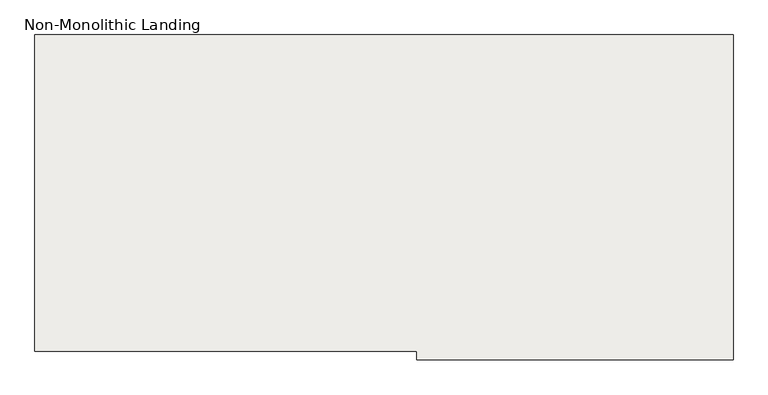
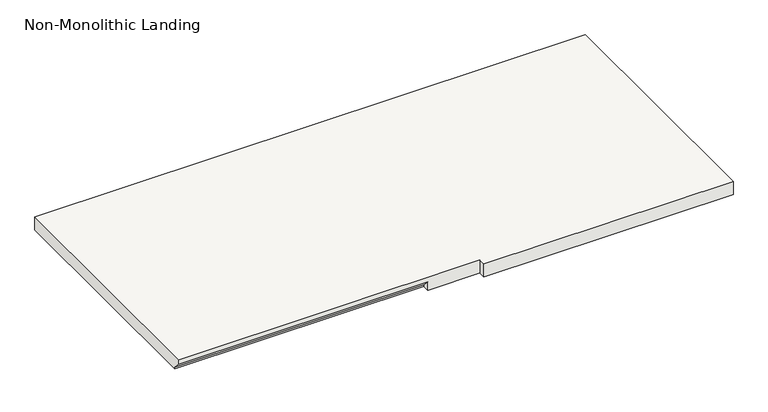
"""IFC4 building model written with IfcOpenShell, lengths in millimetres: slab geometry, Non-Monolithic Landing."""

from ifc_helpers import new_model, si_unit, origin, place, context, project, spatial, faceted_brep, source, transform, mapped, element, save


def non_monolithic_landing_4d8e9abd(model_context):
    return source(origin(), model_context, "Body", "Brep", [
        faceted_brep([(-12643.368339, 8412.443496, 8591.55), (-12643.368339, 8437.843496, 8566.15), (-11728.968339, 8437.843496, 8566.15), (-11728.968339, 8412.443496, 8591.55), (-11538.468339, 8412.443496, 8610.6), (-11538.468339, 8387.043496, 8610.6), (-10624.068339, 8387.043496, 8610.6), (-10624.068339, 8412.443496, 8610.6), (-10624.068339, 9326.843496, 8610.6), (-12643.368339, 9326.843496, 8610.6), (-12643.368339, 8412.443496, 8610.6), (-11728.968339, 8437.843496, 8559.8), (-12643.368339, 8437.843496, 8559.8), (-12643.368339, 9326.843496, 8559.8), (-10624.068339, 9326.843496, 8559.8), (-10624.068339, 8412.443496, 8559.8), (-10624.068339, 8387.043496, 8559.8), (-11538.468339, 8387.043496, 8559.8), (-11538.468339, 8412.443496, 8559.8), (-11728.968339, 8412.443496, 8559.8)], [[[0, 1, 2, 3]], [[4, 5, 6, 7, 8, 9, 10]], [[11, 12, 13, 14, 15, 16, 17, 18, 19]], [[12, 11, 2, 1]], [[11, 19, 3, 2]], [[4, 10, 0, 3, 19, 18]], [[5, 4, 18, 17]], [[6, 5, 17, 16]], [[7, 6, 16, 15]], [[8, 7, 15, 14]], [[9, 8, 14, 13]], [[10, 9, 13, 12, 1, 0]]]),
    ])


if __name__ == "__main__":
    model = new_model("IFC4")
    model_context = context("Model", 3, world=origin())
    ifc_project = project(units=[si_unit("LENGTHUNIT", "METRE", prefix="MILLI")], contexts=[model_context])
    site = spatial("IfcSite", under=ifc_project)
    building = spatial("IfcBuilding", under=site)
    placement = place(None, origin())
    non_monolithic_landing_shape = non_monolithic_landing_4d8e9abd(model_context)
    element("IfcSlab", 1, ObjectType="Non-Monolithic Landing", at=placement, inside=building, context=model_context, shape_type="MappedRepresentation", body=[
        mapped(non_monolithic_landing_shape, transform((0.0, 0.0, 0.0), x_axis=(1.0, 0.0, 0.0), y_axis=(0.0, 1.0, 0.0), z_axis=(0.0, 0.0, 1.0))),
    ])
    save(model, "model.ifc")
